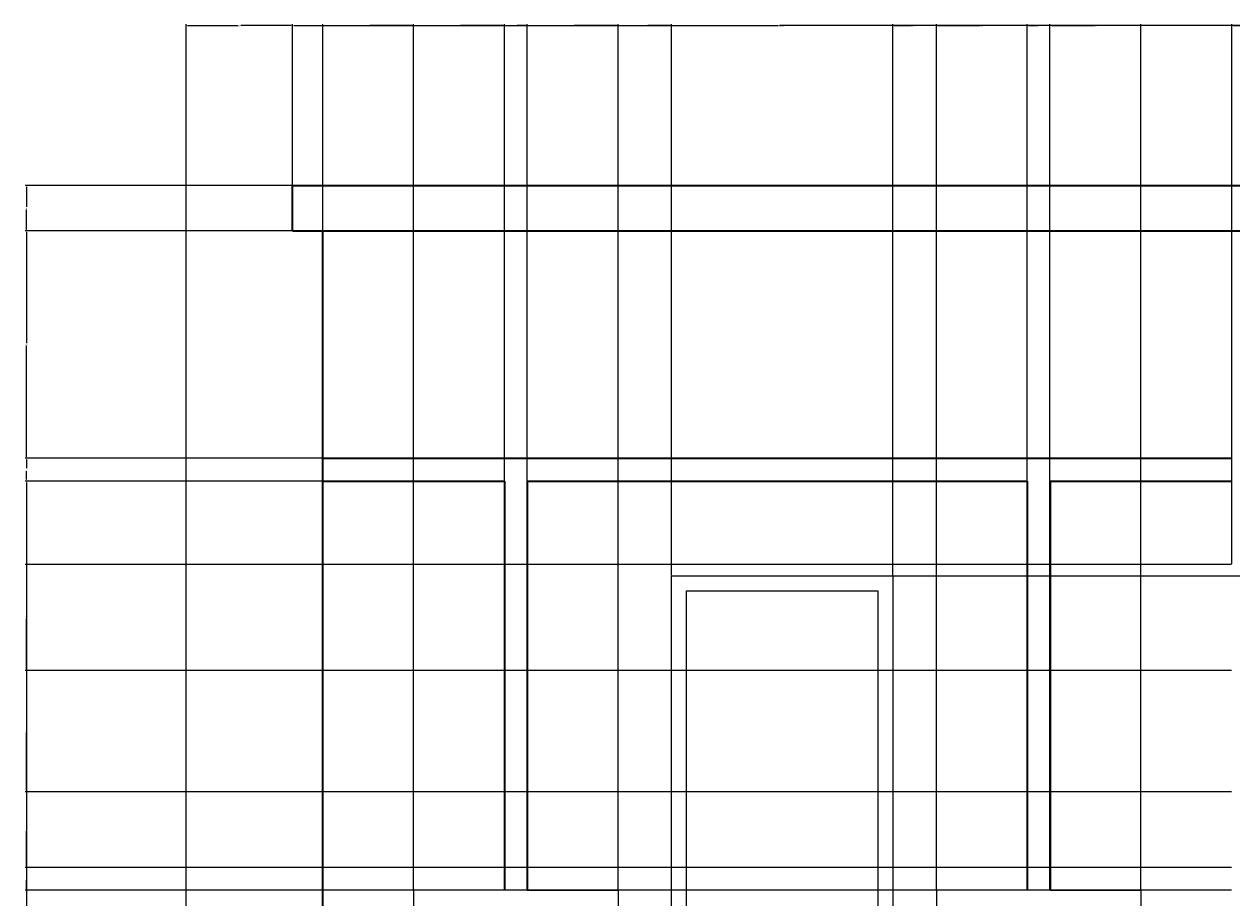
# Model space of a CAD drawing. Units: inches. Extents: x 2148 to 2587, y 1015 to 1466.
# Tile 5 of 7: x 2148 to 2307, y 1351 to 1466. Entities that reach past the tile are written whole.
import ezdxf

# ---------------------------------------------------------------- set-up
doc = ezdxf.new("R2010")
doc.units = ezdxf.units.IN
for name, color, linetype, lineweight in [('A-ANNO-DIMS', 2, 'Continuous', 18), ('A-ELEV', 7, 'Continuous', 35), ('A-GLAZ', 4, 'Continuous', 25)]:
    doc.layers.add(name, color=color, linetype=linetype, lineweight=lineweight)
doc.styles.get("Standard").update_dxf_attribs({"font": 'arial.ttf'})
doc.dimstyles.get("Standard").update_dxf_attribs({"dimtxt": 0.18, "dimasz": 0.18, "dimexe": 0.18, "dimexo": 0.0625, "dimgap": 0.09, "dimtad": 0, "dimtih": 1, "dimtoh": 1, "dimdec": 4, "dimzin": 0, "dimdsep": 46, "dimtxsty": 'Standard', "dimcen": 0.09, "dimadec": 0, "dimazin": 0, "dimtfac": 1, "dimtdec": 4, "dimtofl": 0, "dimtmove": 0, "dimatfit": 3, "dimfxl": 1, "dimtolj": 1, "dimtzin": 0, "dimarcsym": 0})

# ---------------------------------------------------------------- blocks, each defined once
blk = doc.blocks.new('*D7')
at = {"layer": 'A-ANNO-DIMS', "color": 0, "lineweight": -2, "transparency": 16777216}
for p, q in [((2169.03, 1305.54), (2169.03, 1466.02)), ((2169.21, 1465.84), (2175.82, 1465.84)), ((2182.85, 1465.84), (2176.24, 1465.84)), ((2183.03, 1444.81), (2183.03, 1466.02))]:
    blk.add_line(p, q, dxfattribs=at)
at = {"layer": 'A-ANNO-DIMS', "color": 0, "transparency": 16777216}
for points in [[(2169.21, 1465.87), (2169.21, 1465.81), (2169.03, 1465.84)], [(2182.85, 1465.87), (2182.85, 1465.81), (2183.03, 1465.84)]]:
    blk.add_solid(points, dxfattribs=at)
at = {"layer": 'Defpoints', "color": 0, "transparency": 16777216}
for p in [(2183.03, 1465.84), (2183.03, 1444.74), (2169.03, 1305.47)]:
    blk.add_point(p, dxfattribs=at)
at = {"layer": 'A-ANNO-DIMS', "color": 0, "transparency": 16777216, "insert": (2176.03, 1465.84), "char_height": 0.18, "attachment_point": 5}
blk.add_mtext('\\A1;14', dxfattribs=at)
blk = doc.blocks.new('*D8')
at = {"layer": 'A-ANNO-DIMS', "color": 0, "lineweight": -2, "transparency": 16777216}
for p, q in [((2183.03, 1444.81), (2183.03, 1466.02)), ((2183.21, 1465.84), (2246.75, 1465.84)), ((2310.85, 1465.84), (2247.31, 1465.84)), ((2311.03, 1444.81), (2311.03, 1466.02))]:
    blk.add_line(p, q, dxfattribs=at)
at = {"layer": 'A-ANNO-DIMS', "color": 0, "transparency": 16777216}
for points in [[(2183.21, 1465.87), (2183.21, 1465.81), (2183.03, 1465.84)], [(2310.85, 1465.87), (2310.85, 1465.81), (2311.03, 1465.84)]]:
    blk.add_solid(points, dxfattribs=at)
at = {"layer": 'Defpoints', "color": 0, "transparency": 16777216}
for p in [(2311.03, 1465.84), (2183.03, 1444.74), (2311.03, 1444.74)]:
    blk.add_point(p, dxfattribs=at)
at = {"layer": 'A-ANNO-DIMS', "color": 0, "transparency": 16777216, "insert": (2247.03, 1465.84), "char_height": 0.18, "attachment_point": 5}
blk.add_mtext('\\A1;128', dxfattribs=at)
blk = doc.blocks.new('*D23')
at = {"layer": 'A-ANNO-DIMS', "color": 0, "lineweight": -2, "transparency": 16777216}
for p, q in [((2186.97, 1405.74), (2147.75, 1405.74)), ((2147.93, 1405.56), (2147.93, 1286.42)), ((2147.93, 1166.92), (2147.93, 1286.06)), ((2186.97, 1166.74), (2147.75, 1166.74))]:
    blk.add_line(p, q, dxfattribs=at)
at = {"layer": 'A-ANNO-DIMS', "color": 0, "transparency": 16777216}
for points in [[(2147.9, 1405.56), (2147.96, 1405.56), (2147.93, 1405.74)], [(2147.9, 1166.92), (2147.96, 1166.92), (2147.93, 1166.74)]]:
    blk.add_solid(points, dxfattribs=at)
at = {"layer": 'Defpoints', "color": 0, "transparency": 16777216}
for p in [(2147.93, 1405.74), (2187.03, 1405.74), (2187.03, 1166.74)]:
    blk.add_point(p, dxfattribs=at)
at = {"layer": 'A-ANNO-DIMS', "color": 0, "transparency": 16777216, "insert": (2147.93, 1286.24), "char_height": 0.18, "attachment_point": 5}
blk.add_mtext('\\A1;239', dxfattribs=at)
blk = doc.blocks.new('*D24')
at = {"layer": 'A-ANNO-DIMS', "color": 0, "lineweight": -2, "transparency": 16777216}
for p, q in [((2186.97, 1408.74), (2147.75, 1408.74)), ((2147.93, 1408.56), (2147.93, 1407.42)), ((2147.93, 1405.92), (2147.93, 1407.06)), ((2186.97, 1405.74), (2147.75, 1405.74))]:
    blk.add_line(p, q, dxfattribs=at)
at = {"layer": 'A-ANNO-DIMS', "color": 0, "transparency": 16777216}
for points in [[(2147.9, 1408.56), (2147.96, 1408.56), (2147.93, 1408.74)], [(2147.9, 1405.92), (2147.96, 1405.92), (2147.93, 1405.74)]]:
    blk.add_solid(points, dxfattribs=at)
at = {"layer": 'Defpoints', "color": 0, "transparency": 16777216}
for p in [(2147.93, 1408.74), (2187.03, 1408.74), (2187.03, 1405.74)]:
    blk.add_point(p, dxfattribs=at)
at = {"layer": 'A-ANNO-DIMS', "color": 0, "transparency": 16777216, "insert": (2147.93, 1407.24), "char_height": 0.18, "attachment_point": 5}
blk.add_mtext('\\A1;3', dxfattribs=at)
blk = doc.blocks.new('*D25')
at = {"layer": 'A-ANNO-DIMS', "color": 0, "lineweight": -2, "transparency": 16777216}
for p, q in [((2182.97, 1438.74), (2147.75, 1438.74)), ((2147.93, 1438.56), (2147.93, 1423.92)), ((2147.93, 1408.92), (2147.93, 1423.56)), ((2186.97, 1408.74), (2147.75, 1408.74))]:
    blk.add_line(p, q, dxfattribs=at)
at = {"layer": 'A-ANNO-DIMS', "color": 0, "transparency": 16777216}
for points in [[(2147.9, 1438.56), (2147.96, 1438.56), (2147.93, 1438.74)], [(2147.9, 1408.92), (2147.96, 1408.92), (2147.93, 1408.74)]]:
    blk.add_solid(points, dxfattribs=at)
at = {"layer": 'Defpoints', "color": 0, "transparency": 16777216}
for p in [(2147.93, 1438.74), (2183.03, 1438.74), (2187.03, 1408.74)]:
    blk.add_point(p, dxfattribs=at)
at = {"layer": 'A-ANNO-DIMS', "color": 0, "transparency": 16777216, "insert": (2147.93, 1423.74), "char_height": 0.18, "attachment_point": 5}
blk.add_mtext('\\A1;30', dxfattribs=at)
blk = doc.blocks.new('*D26')
at = {"layer": 'A-ANNO-DIMS', "color": 0, "lineweight": -2, "transparency": 16777216}
for p, q in [((2182.97, 1444.74), (2147.75, 1444.74)), ((2147.93, 1444.56), (2147.93, 1441.92)), ((2147.93, 1438.92), (2147.93, 1441.56)), ((2182.97, 1438.74), (2147.75, 1438.74))]:
    blk.add_line(p, q, dxfattribs=at)
at = {"layer": 'A-ANNO-DIMS', "color": 0, "transparency": 16777216}
for points in [[(2147.9, 1444.56), (2147.96, 1444.56), (2147.93, 1444.74)], [(2147.9, 1438.92), (2147.96, 1438.92), (2147.93, 1438.74)]]:
    blk.add_solid(points, dxfattribs=at)
at = {"layer": 'Defpoints', "color": 0, "transparency": 16777216}
for p in [(2147.93, 1444.74), (2183.03, 1444.74), (2183.03, 1438.74)]:
    blk.add_point(p, dxfattribs=at)
at = {"layer": 'A-ANNO-DIMS', "color": 0, "transparency": 16777216, "insert": (2147.93, 1441.74), "char_height": 0.18, "attachment_point": 5}
blk.add_mtext('\\A1;6', dxfattribs=at)
blk = doc.blocks.new('*D33')
at = {"layer": 'A-ANNO-DIMS', "color": 0, "lineweight": -2, "transparency": 16777216}
for p, q in [((2307.03, 1394.81), (2307.03, 1466.02)), ((2307.21, 1465.84), (2324.89, 1465.84)), ((2343.5, 1465.84), (2325.82, 1465.84)), ((2343.68, 1366.81), (2343.68, 1466.02))]:
    blk.add_line(p, q, dxfattribs=at)
at = {"layer": 'A-ANNO-DIMS', "color": 0, "transparency": 16777216}
for points in [[(2307.21, 1465.87), (2307.21, 1465.81), (2307.03, 1465.84)], [(2343.5, 1465.87), (2343.5, 1465.81), (2343.68, 1465.84)]]:
    blk.add_solid(points, dxfattribs=at)
at = {"layer": 'Defpoints', "color": 0, "transparency": 16777216}
for p in [(2343.68, 1465.84), (2307.03, 1394.74), (2343.68, 1366.74)]:
    blk.add_point(p, dxfattribs=at)
at = {"layer": 'A-ANNO-DIMS', "color": 0, "transparency": 16777216, "insert": (2325.36, 1465.84), "char_height": 0.18, "attachment_point": 5}
blk.add_mtext('\\A1;36.645', dxfattribs=at)
blk = doc.blocks.new('*D66')
at = {"layer": 'A-ANNO-DIMS', "color": 0, "lineweight": -2, "transparency": 16777216}
for p, q in [((2306.97, 1351.74), (2147.75, 1351.74)), ((2147.93, 1351.56), (2147.93, 1349.42)), ((2147.93, 1346.92), (2147.93, 1349.06)), ((2306.97, 1346.74), (2147.75, 1346.74))]:
    blk.add_line(p, q, dxfattribs=at)
at = {"layer": 'A-ANNO-DIMS', "color": 0, "transparency": 16777216}
for points in [[(2147.9, 1351.56), (2147.96, 1351.56), (2147.93, 1351.74)], [(2147.9, 1346.92), (2147.96, 1346.92), (2147.93, 1346.74)]]:
    blk.add_solid(points, dxfattribs=at)
at = {"layer": 'Defpoints', "color": 0, "transparency": 16777216}
for p in [(2147.93, 1351.74), (2307.03, 1351.74), (2307.03, 1346.74)]:
    blk.add_point(p, dxfattribs=at)
at = {"layer": 'A-ANNO-DIMS', "color": 0, "transparency": 16777216, "insert": (2147.93, 1349.24), "char_height": 0.18, "attachment_point": 5}
blk.add_mtext('\\A1;5', dxfattribs=at)
blk = doc.blocks.new('*D67')
at = {"layer": 'A-ANNO-DIMS', "color": 0, "lineweight": -2, "transparency": 16777216}
for p, q in [((2306.97, 1354.74), (2147.75, 1354.74)), ((2147.93, 1354.56), (2147.93, 1353.42)), ((2147.93, 1351.92), (2147.93, 1353.06)), ((2306.97, 1351.74), (2147.75, 1351.74))]:
    blk.add_line(p, q, dxfattribs=at)
at = {"layer": 'A-ANNO-DIMS', "color": 0, "transparency": 16777216}
for points in [[(2147.9, 1354.56), (2147.96, 1354.56), (2147.93, 1354.74)], [(2147.9, 1351.92), (2147.96, 1351.92), (2147.93, 1351.74)]]:
    blk.add_solid(points, dxfattribs=at)
at = {"layer": 'Defpoints', "color": 0, "transparency": 16777216}
for p in [(2147.93, 1354.74), (2307.03, 1354.74), (2307.03, 1351.74)]:
    blk.add_point(p, dxfattribs=at)
at = {"layer": 'A-ANNO-DIMS', "color": 0, "transparency": 16777216, "insert": (2147.93, 1353.24), "char_height": 0.18, "attachment_point": 5}
blk.add_mtext('\\A1;3', dxfattribs=at)
blk = doc.blocks.new('*D68')
at = {"layer": 'A-ANNO-DIMS', "color": 0, "lineweight": -2, "transparency": 16777216}
for p, q in [((2306.97, 1364.74), (2147.75, 1364.74)), ((2147.93, 1364.56), (2147.93, 1359.92)), ((2147.93, 1354.92), (2147.93, 1359.56)), ((2306.97, 1354.74), (2147.75, 1354.74))]:
    blk.add_line(p, q, dxfattribs=at)
at = {"layer": 'A-ANNO-DIMS', "color": 0, "transparency": 16777216}
for points in [[(2147.9, 1364.56), (2147.96, 1364.56), (2147.93, 1364.74)], [(2147.9, 1354.92), (2147.96, 1354.92), (2147.93, 1354.74)]]:
    blk.add_solid(points, dxfattribs=at)
at = {"layer": 'Defpoints', "color": 0, "transparency": 16777216}
for p in [(2147.93, 1364.74), (2307.03, 1364.74), (2307.03, 1354.74)]:
    blk.add_point(p, dxfattribs=at)
at = {"layer": 'A-ANNO-DIMS', "color": 0, "transparency": 16777216, "insert": (2147.93, 1359.74), "char_height": 0.18, "attachment_point": 5}
blk.add_mtext('\\A1;10', dxfattribs=at)
blk = doc.blocks.new('*D69')
at = {"layer": 'A-ANNO-DIMS', "color": 0, "lineweight": -2, "transparency": 16777216}
for p, q in [((2306.97, 1380.74), (2147.75, 1380.74)), ((2147.93, 1380.56), (2147.93, 1372.92)), ((2147.93, 1364.92), (2147.93, 1372.56)), ((2306.97, 1364.74), (2147.75, 1364.74))]:
    blk.add_line(p, q, dxfattribs=at)
at = {"layer": 'A-ANNO-DIMS', "color": 0, "transparency": 16777216}
for points in [[(2147.9, 1380.56), (2147.96, 1380.56), (2147.93, 1380.74)], [(2147.9, 1364.92), (2147.96, 1364.92), (2147.93, 1364.74)]]:
    blk.add_solid(points, dxfattribs=at)
at = {"layer": 'Defpoints', "color": 0, "transparency": 16777216}
for p in [(2147.93, 1380.74), (2307.03, 1380.74), (2307.03, 1364.74)]:
    blk.add_point(p, dxfattribs=at)
at = {"layer": 'A-ANNO-DIMS', "color": 0, "transparency": 16777216, "insert": (2147.93, 1372.74), "char_height": 0.18, "attachment_point": 5}
blk.add_mtext('\\A1;16', dxfattribs=at)
blk = doc.blocks.new('*D70')
at = {"layer": 'A-ANNO-DIMS', "color": 0, "lineweight": -2, "transparency": 16777216}
for p, q in [((2306.97, 1394.74), (2147.75, 1394.74)), ((2147.93, 1394.56), (2147.93, 1387.92)), ((2147.93, 1380.92), (2147.93, 1387.56)), ((2306.97, 1380.74), (2147.75, 1380.74))]:
    blk.add_line(p, q, dxfattribs=at)
at = {"layer": 'A-ANNO-DIMS', "color": 0, "transparency": 16777216}
for points in [[(2147.9, 1394.56), (2147.96, 1394.56), (2147.93, 1394.74)], [(2147.9, 1380.92), (2147.96, 1380.92), (2147.93, 1380.74)]]:
    blk.add_solid(points, dxfattribs=at)
at = {"layer": 'Defpoints', "color": 0, "transparency": 16777216}
for p in [(2147.93, 1394.74), (2307.03, 1394.74), (2307.03, 1380.74)]:
    blk.add_point(p, dxfattribs=at)
at = {"layer": 'A-ANNO-DIMS', "color": 0, "transparency": 16777216, "insert": (2147.93, 1387.74), "char_height": 0.18, "attachment_point": 5}
blk.add_mtext('\\A1;14', dxfattribs=at)
blk = doc.blocks.new('*D73')
at = {"layer": 'A-ANNO-DIMS', "color": 0, "lineweight": -2, "transparency": 16777216}
for p, q in [((2187.03, 1166.81), (2187.03, 1466.02)), ((2187.21, 1465.84), (2192.82, 1465.84)), ((2198.85, 1465.84), (2193.24, 1465.84)), ((2199.03, 1351.81), (2199.03, 1466.02))]:
    blk.add_line(p, q, dxfattribs=at)
at = {"layer": 'A-ANNO-DIMS', "color": 0, "transparency": 16777216}
for points in [[(2187.21, 1465.87), (2187.21, 1465.81), (2187.03, 1465.84)], [(2198.85, 1465.87), (2198.85, 1465.81), (2199.03, 1465.84)]]:
    blk.add_solid(points, dxfattribs=at)
at = {"layer": 'Defpoints', "color": 0, "transparency": 16777216}
for p in [(2199.03, 1465.84), (2199.03, 1351.74), (2187.03, 1166.74)]:
    blk.add_point(p, dxfattribs=at)
at = {"layer": 'A-ANNO-DIMS', "color": 0, "transparency": 16777216, "insert": (2193.03, 1465.84), "char_height": 0.18, "attachment_point": 5}
blk.add_mtext('\\A1;12', dxfattribs=at)
blk = doc.blocks.new('*D74')
at = {"layer": 'A-ANNO-DIMS', "color": 0, "lineweight": -2, "transparency": 16777216}
for p, q in [((2199.03, 1351.81), (2199.03, 1466.02)), ((2199.21, 1465.84), (2204.82, 1465.84)), ((2210.85, 1465.84), (2205.24, 1465.84)), ((2211.03, 1351.81), (2211.03, 1466.02))]:
    blk.add_line(p, q, dxfattribs=at)
at = {"layer": 'A-ANNO-DIMS', "color": 0, "transparency": 16777216}
for points in [[(2199.21, 1465.87), (2199.21, 1465.81), (2199.03, 1465.84)], [(2210.85, 1465.87), (2210.85, 1465.81), (2211.03, 1465.84)]]:
    blk.add_solid(points, dxfattribs=at)
at = {"layer": 'Defpoints', "color": 0, "transparency": 16777216}
for p in [(2211.03, 1465.84), (2199.03, 1351.74), (2211.03, 1351.74)]:
    blk.add_point(p, dxfattribs=at)
at = {"layer": 'A-ANNO-DIMS', "color": 0, "transparency": 16777216, "insert": (2205.03, 1465.84), "char_height": 0.18, "attachment_point": 5}
blk.add_mtext('\\A1;12', dxfattribs=at)
blk = doc.blocks.new('*D75')
at = {"layer": 'A-ANNO-DIMS', "color": 0, "lineweight": -2, "transparency": 16777216}
for p, q in [((2211.03, 1351.81), (2211.03, 1466.02)), ((2211.21, 1465.84), (2212.39, 1465.84)), ((2213.85, 1465.84), (2212.68, 1465.84)), ((2214.03, 1351.81), (2214.03, 1466.02))]:
    blk.add_line(p, q, dxfattribs=at)
at = {"layer": 'A-ANNO-DIMS', "color": 0, "transparency": 16777216}
for points in [[(2211.21, 1465.87), (2211.21, 1465.81), (2211.03, 1465.84)], [(2213.85, 1465.87), (2213.85, 1465.81), (2214.03, 1465.84)]]:
    blk.add_solid(points, dxfattribs=at)
at = {"layer": 'Defpoints', "color": 0, "transparency": 16777216}
for p in [(2214.03, 1465.84), (2211.03, 1351.74), (2214.03, 1351.74)]:
    blk.add_point(p, dxfattribs=at)
at = {"layer": 'A-ANNO-DIMS', "color": 0, "transparency": 16777216, "insert": (2212.53, 1465.84), "char_height": 0.18, "attachment_point": 5}
blk.add_mtext('\\A1;3', dxfattribs=at)
blk = doc.blocks.new('*D76')
at = {"layer": 'A-ANNO-DIMS', "color": 0, "lineweight": -2, "transparency": 16777216}
for p, q in [((2214.03, 1351.81), (2214.03, 1466.02)), ((2214.21, 1465.84), (2219.82, 1465.84)), ((2225.85, 1465.84), (2220.24, 1465.84)), ((2226.03, 1351.81), (2226.03, 1466.02))]:
    blk.add_line(p, q, dxfattribs=at)
at = {"layer": 'A-ANNO-DIMS', "color": 0, "transparency": 16777216}
for points in [[(2214.21, 1465.87), (2214.21, 1465.81), (2214.03, 1465.84)], [(2225.85, 1465.87), (2225.85, 1465.81), (2226.03, 1465.84)]]:
    blk.add_solid(points, dxfattribs=at)
at = {"layer": 'Defpoints', "color": 0, "transparency": 16777216}
for p in [(2226.03, 1465.84), (2214.03, 1351.74), (2226.03, 1351.74)]:
    blk.add_point(p, dxfattribs=at)
at = {"layer": 'A-ANNO-DIMS', "color": 0, "transparency": 16777216, "insert": (2220.03, 1465.84), "char_height": 0.18, "attachment_point": 5}
blk.add_mtext('\\A1;12', dxfattribs=at)
blk = doc.blocks.new('*D77')
at = {"layer": 'A-ANNO-DIMS', "color": 0, "lineweight": -2, "transparency": 16777216}
for p, q in [((2226.03, 1351.81), (2226.03, 1466.02)), ((2226.21, 1465.84), (2229.15, 1465.84)), ((2232.88, 1465.84), (2229.94, 1465.84)), ((2233.06, 1393.3), (2233.06, 1466.02))]:
    blk.add_line(p, q, dxfattribs=at)
at = {"layer": 'A-ANNO-DIMS', "color": 0, "transparency": 16777216}
for points in [[(2226.21, 1465.87), (2226.21, 1465.81), (2226.03, 1465.84)], [(2232.88, 1465.87), (2232.88, 1465.81), (2233.06, 1465.84)]]:
    blk.add_solid(points, dxfattribs=at)
at = {"layer": 'Defpoints', "color": 0, "transparency": 16777216}
for p in [(2233.06, 1465.84), (2233.06, 1393.24), (2226.03, 1351.74)]:
    blk.add_point(p, dxfattribs=at)
at = {"layer": 'A-ANNO-DIMS', "color": 0, "transparency": 16777216, "insert": (2229.55, 1465.84), "char_height": 0.18, "attachment_point": 5}
blk.add_mtext('\\A1;7.026', dxfattribs=at)
blk = doc.blocks.new('*D78')
at = {"layer": 'A-ANNO-DIMS', "color": 0, "lineweight": -2, "transparency": 16777216}
for p, q in [((2233.06, 1393.3), (2233.06, 1466.02)), ((2233.24, 1465.84), (2247.21, 1465.84)), ((2262.11, 1465.84), (2248.14, 1465.84)), ((2262.29, 1393.3), (2262.29, 1466.02))]:
    blk.add_line(p, q, dxfattribs=at)
at = {"layer": 'A-ANNO-DIMS', "color": 0, "transparency": 16777216}
for points in [[(2233.24, 1465.87), (2233.24, 1465.81), (2233.06, 1465.84)], [(2262.11, 1465.87), (2262.11, 1465.81), (2262.29, 1465.84)]]:
    blk.add_solid(points, dxfattribs=at)
at = {"layer": 'Defpoints', "color": 0, "transparency": 16777216}
for p in [(2262.29, 1465.84), (2233.06, 1393.24), (2262.29, 1393.24)]:
    blk.add_point(p, dxfattribs=at)
at = {"layer": 'A-ANNO-DIMS', "color": 0, "transparency": 16777216, "insert": (2247.67, 1465.84), "char_height": 0.18, "attachment_point": 5}
blk.add_mtext('\\A1;29.227', dxfattribs=at)
blk = doc.blocks.new('*D79')
at = {"layer": 'A-ANNO-DIMS', "color": 0, "lineweight": -2, "transparency": 16777216}
for p, q in [((2262.29, 1393.3), (2262.29, 1466.02)), ((2262.47, 1465.84), (2264.77, 1465.84)), ((2267.85, 1465.84), (2265.55, 1465.84)), ((2268.03, 1351.81), (2268.03, 1466.02))]:
    blk.add_line(p, q, dxfattribs=at)
at = {"layer": 'A-ANNO-DIMS', "color": 0, "transparency": 16777216}
for points in [[(2262.47, 1465.87), (2262.47, 1465.81), (2262.29, 1465.84)], [(2267.85, 1465.87), (2267.85, 1465.81), (2268.03, 1465.84)]]:
    blk.add_solid(points, dxfattribs=at)
at = {"layer": 'Defpoints', "color": 0, "transparency": 16777216}
for p in [(2268.03, 1465.84), (2262.29, 1393.24), (2268.03, 1351.74)]:
    blk.add_point(p, dxfattribs=at)
at = {"layer": 'A-ANNO-DIMS', "color": 0, "transparency": 16777216, "insert": (2265.16, 1465.84), "char_height": 0.18, "attachment_point": 5}
blk.add_mtext('\\A1;5.747', dxfattribs=at)
blk = doc.blocks.new('*D80')
at = {"layer": 'A-ANNO-DIMS', "color": 0, "lineweight": -2, "transparency": 16777216}
for p, q in [((2268.03, 1351.81), (2268.03, 1466.02)), ((2268.21, 1465.84), (2273.82, 1465.84)), ((2279.85, 1465.84), (2274.24, 1465.84)), ((2280.03, 1351.81), (2280.03, 1466.02))]:
    blk.add_line(p, q, dxfattribs=at)
at = {"layer": 'A-ANNO-DIMS', "color": 0, "transparency": 16777216}
for points in [[(2268.21, 1465.87), (2268.21, 1465.81), (2268.03, 1465.84)], [(2279.85, 1465.87), (2279.85, 1465.81), (2280.03, 1465.84)]]:
    blk.add_solid(points, dxfattribs=at)
at = {"layer": 'Defpoints', "color": 0, "transparency": 16777216}
for p in [(2280.03, 1465.84), (2268.03, 1351.74), (2280.03, 1351.74)]:
    blk.add_point(p, dxfattribs=at)
at = {"layer": 'A-ANNO-DIMS', "color": 0, "transparency": 16777216, "insert": (2274.03, 1465.84), "char_height": 0.18, "attachment_point": 5}
blk.add_mtext('\\A1;12', dxfattribs=at)
blk = doc.blocks.new('*D81')
at = {"layer": 'A-ANNO-DIMS', "color": 0, "lineweight": -2, "transparency": 16777216}
for p, q in [((2280.03, 1351.81), (2280.03, 1466.02)), ((2280.21, 1465.84), (2281.39, 1465.84)), ((2282.85, 1465.84), (2281.68, 1465.84)), ((2283.03, 1351.81), (2283.03, 1466.02))]:
    blk.add_line(p, q, dxfattribs=at)
at = {"layer": 'A-ANNO-DIMS', "color": 0, "transparency": 16777216}
for points in [[(2280.21, 1465.87), (2280.21, 1465.81), (2280.03, 1465.84)], [(2282.85, 1465.87), (2282.85, 1465.81), (2283.03, 1465.84)]]:
    blk.add_solid(points, dxfattribs=at)
at = {"layer": 'Defpoints', "color": 0, "transparency": 16777216}
for p in [(2283.03, 1465.84), (2280.03, 1351.74), (2283.03, 1351.74)]:
    blk.add_point(p, dxfattribs=at)
at = {"layer": 'A-ANNO-DIMS', "color": 0, "transparency": 16777216, "insert": (2281.53, 1465.84), "char_height": 0.18, "attachment_point": 5}
blk.add_mtext('\\A1;3', dxfattribs=at)
blk = doc.blocks.new('*D82')
at = {"layer": 'A-ANNO-DIMS', "color": 0, "lineweight": -2, "transparency": 16777216}
for p, q in [((2283.03, 1351.81), (2283.03, 1466.02)), ((2283.21, 1465.84), (2288.82, 1465.84)), ((2294.85, 1465.84), (2289.24, 1465.84)), ((2295.03, 1351.81), (2295.03, 1466.02))]:
    blk.add_line(p, q, dxfattribs=at)
at = {"layer": 'A-ANNO-DIMS', "color": 0, "transparency": 16777216}
for points in [[(2283.21, 1465.87), (2283.21, 1465.81), (2283.03, 1465.84)], [(2294.85, 1465.87), (2294.85, 1465.81), (2295.03, 1465.84)]]:
    blk.add_solid(points, dxfattribs=at)
at = {"layer": 'Defpoints', "color": 0, "transparency": 16777216}
for p in [(2295.03, 1465.84), (2283.03, 1351.74), (2295.03, 1351.74)]:
    blk.add_point(p, dxfattribs=at)
at = {"layer": 'A-ANNO-DIMS', "color": 0, "transparency": 16777216, "insert": (2289.03, 1465.84), "char_height": 0.18, "attachment_point": 5}
blk.add_mtext('\\A1;12', dxfattribs=at)
blk = doc.blocks.new('*D91')
at = {"layer": 'A-ANNO-DIMS', "color": 0, "lineweight": -2, "transparency": 16777216}
for p, q in [((2198.97, 1351.74), (2147.75, 1351.74)), ((2147.93, 1351.56), (2147.93, 1269.82)), ((2147.93, 1187.71), (2147.93, 1269.45)), ((2201.43, 1187.53), (2147.75, 1187.53))]:
    blk.add_line(p, q, dxfattribs=at)
at = {"layer": 'A-ANNO-DIMS', "color": 0, "transparency": 16777216}
for points in [[(2147.9, 1351.56), (2147.96, 1351.56), (2147.93, 1351.74)], [(2147.9, 1187.71), (2147.96, 1187.71), (2147.93, 1187.53)]]:
    blk.add_solid(points, dxfattribs=at)
at = {"layer": 'Defpoints', "color": 0, "transparency": 16777216}
for p in [(2147.93, 1351.74), (2199.03, 1351.74), (2201.49, 1187.53)]:
    blk.add_point(p, dxfattribs=at)
at = {"layer": 'A-ANNO-DIMS', "color": 0, "transparency": 16777216, "insert": (2147.93, 1269.64), "char_height": 0.18, "attachment_point": 5}
blk.add_mtext('\\A1;164.2', dxfattribs=at)
blk = doc.blocks.new('*D97')
at = {"layer": 'A-ANNO-DIMS', "color": 0, "lineweight": -2, "transparency": 16777216}
for p, q in [((2262.35, 1393.24), (2586.31, 1393.24)), ((2586.13, 1393.06), (2586.13, 1369.55)), ((2586.13, 1345.67), (2586.13, 1369.18)), ((2260.35, 1345.49), (2586.31, 1345.49))]:
    blk.add_line(p, q, dxfattribs=at)
at = {"layer": 'A-ANNO-DIMS', "color": 0, "transparency": 16777216}
for points in [[(2586.1, 1393.06), (2586.16, 1393.06), (2586.13, 1393.24)], [(2586.1, 1345.67), (2586.16, 1345.67), (2586.13, 1345.49)]]:
    blk.add_solid(points, dxfattribs=at)
at = {"layer": 'Defpoints', "color": 0, "transparency": 16777216}
for p in [(2262.29, 1393.24), (2586.13, 1393.24), (2260.29, 1345.49)]:
    blk.add_point(p, dxfattribs=at)
at = {"layer": 'A-ANNO-DIMS', "color": 0, "transparency": 16777216, "insert": (2586.13, 1369.36), "char_height": 0.18, "attachment_point": 5}
blk.add_mtext('\\A1;47.75', dxfattribs=at)

msp = doc.modelspace()

# ---------------------------------------------------------------- linework, layer by layer
at = {"layer": 'A-ELEV'}
for p, q in [((2183.0343, 1438.7427), (2183.0343, 1444.7427)), ((2183.0343, 1444.7427), (2311.0343, 1444.7427)), ((2183.0343, 1438.7427), (2311.0343, 1438.7427)), ((2187.0343, 1048.7427), (2187.0343, 1438.7427)), ((2187.0343, 1408.7427), (2307.0343, 1408.7427)), ((2187.0343, 1405.7427), (2211.0343, 1405.7427)), ((2211.0343, 1405.7427), (2211.0343, 1351.7427)), ((2214.0343, 1405.7427), (2214.0343, 1351.7427)), ((2214.0343, 1405.7427), (2280.0343, 1405.7427)), ((2280.0343, 1405.7427), (2280.0343, 1351.7427)), ((2283.0343, 1405.7427), (2283.0343, 1351.7427)), ((2283.0343, 1405.7427), (2307.0343, 1405.7427))]:
    msp.add_line(p, q, dxfattribs=at)
at = {"layer": 'A-GLAZ'}
for p, q in [((2211.0343, 1351.7427), (2199.0343, 1351.7427)), ((2199.0343, 1351.7427), (2199.0343, 1174.7427)), ((2226.0343, 1351.7427), (2199.0343, 1351.7427)), ((2214.0343, 1351.7427), (2226.0343, 1351.7427)), ((2226.0343, 1351.7427), (2226.0343, 1174.7427)), ((2295.0343, 1351.7427), (2268.0343, 1351.7427)), ((2280.0343, 1351.7427), (2268.0343, 1351.7427)), ((2268.0343, 1351.7427), (2268.0343, 1174.7427)), ((2283.0343, 1351.7427), (2295.0343, 1351.7427)), ((2295.0343, 1351.7427), (2295.0343, 1174.7427))]:
    msp.add_line(p, q, dxfattribs=at)
for points in [[(2262.287, 1197.738), (2233.0602, 1197.738), (2233.0602, 1393.2389), (2262.287, 1393.2389)], [(2260.287, 1199.738), (2235.0602, 1199.738), (2235.0602, 1391.2389), (2260.287, 1391.2389)]]:
    msp.add_lwpolyline(points, close=True, dxfattribs=at)

# ---------------------------------------------------------------- dimensions: what is measured, and where the dimension line sits
at = {"layer": 'A-ANNO-DIMS'}
for base, p1, p2, override, picture, middle in [((2183.0343, 1465.8427), (2169.0343, 1305.4734), (2183.0343, 1444.7427), {"dimdec": 0, "dimlfac": 1, "dimrnd": 0, "dimzin": 0, "dimdsep": 46, "dimlunit": 2}, '*D7', (2176.0343, 1465.8427)), ((2311.0343, 1465.8427), (2183.0343, 1444.7427), (2311.0343, 1444.7427), {"dimdec": 0, "dimlfac": 1, "dimrnd": 0, "dimzin": 0, "dimdsep": 46, "dimlunit": 2}, '*D8', (2247.0343, 1465.8427)), ((2199.0343, 1465.8427), (2187.0343, 1166.7427), (2199.0343, 1351.7427), {"dimdec": 0, "dimlfac": 1, "dimrnd": 0, "dimzin": 0, "dimdsep": 46, "dimlunit": 2}, '*D73', (2193.0343, 1465.8427)), ((2211.0343, 1465.8427), (2199.0343, 1351.7427), (2211.0343, 1351.7427), {"dimdec": 0, "dimlfac": 1, "dimrnd": 0, "dimzin": 0, "dimdsep": 46, "dimlunit": 2}, '*D74', (2205.0343, 1465.8427)), ((2214.0343, 1465.8427), (2211.0343, 1351.7427), (2214.0343, 1351.7427), {"dimdec": 0, "dimlfac": 1, "dimrnd": 0, "dimzin": 0, "dimdsep": 46, "dimlunit": 2}, '*D75', (2212.5343, 1465.8427)), ((2226.0343, 1465.8427), (2214.0343, 1351.7427), (2226.0343, 1351.7427), {"dimdec": 0, "dimlfac": 1, "dimrnd": 0, "dimzin": 0, "dimdsep": 46, "dimlunit": 2}, '*D76', (2220.0343, 1465.8427)), ((2233.0602, 1465.8427), (2226.0343, 1351.7427), (2233.0602, 1393.2389), {"dimdec": 3, "dimlfac": 1, "dimrnd": 0, "dimzin": 0, "dimdsep": 46, "dimlunit": 2}, '*D77', (2229.5472, 1465.8427)), ((2262.287, 1465.8427), (2233.0602, 1393.2389), (2262.287, 1393.2389), {"dimdec": 3, "dimlfac": 1, "dimrnd": 0, "dimzin": 0, "dimdsep": 46, "dimlunit": 2}, '*D78', (2247.6736, 1465.8427)), ((2268.0343, 1465.8427), (2262.287, 1393.2389), (2268.0343, 1351.7427), {"dimdec": 3, "dimlfac": 1, "dimrnd": 0, "dimzin": 0, "dimdsep": 46, "dimlunit": 2}, '*D79', (2265.1606, 1465.8427)), ((2280.0343, 1465.8427), (2268.0343, 1351.7427), (2280.0343, 1351.7427), {"dimdec": 0, "dimlfac": 1, "dimrnd": 0, "dimzin": 0, "dimdsep": 46, "dimlunit": 2}, '*D80', (2274.0343, 1465.8427)), ((2283.0343, 1465.8427), (2280.0343, 1351.7427), (2283.0343, 1351.7427), {"dimdec": 0, "dimlfac": 1, "dimrnd": 0, "dimzin": 0, "dimdsep": 46, "dimlunit": 2}, '*D81', (2281.5343, 1465.8427)), ((2295.0343, 1465.8427), (2283.0343, 1351.7427), (2295.0343, 1351.7427), {"dimdec": 0, "dimlfac": 1, "dimrnd": 0, "dimzin": 0, "dimdsep": 46, "dimlunit": 2}, '*D82', (2289.0343, 1465.8427)), ((2343.6794, 1465.8427), (2307.0343, 1394.7427), (2343.6794, 1366.7427), {"dimdec": 3, "dimlfac": 1, "dimrnd": 0, "dimzin": 0, "dimdsep": 46, "dimlunit": 2}, '*D33', (2325.3568, 1465.8427))]:
    dim = msp.add_linear_dim(base=base, p1=p1, p2=p2, dimstyle='Standard', override=override, dxfattribs=at)
    dim.commit()
    dim.dimension.update_dxf_attribs({"geometry": picture, "text_midpoint": middle})
for base, p1, p2, override, picture, middle in [((2147.9343, 1444.7427), (2183.0343, 1438.7427), (2183.0343, 1444.7427), {"dimdec": 0, "dimlfac": 1, "dimrnd": 0, "dimzin": 0, "dimdsep": 46, "dimlunit": 2}, '*D26', (2147.9343, 1441.7427)), ((2147.9343, 1438.7427), (2187.0343, 1408.7427), (2183.0343, 1438.7427), {"dimdec": 0, "dimlfac": 1, "dimrnd": 0, "dimzin": 0, "dimdsep": 46, "dimlunit": 2}, '*D25', (2147.9343, 1423.7427)), ((2147.9343, 1408.7427), (2187.0343, 1405.7427), (2187.0343, 1408.7427), {"dimdec": 0, "dimlfac": 1, "dimrnd": 0, "dimzin": 0, "dimdsep": 46, "dimlunit": 2}, '*D24', (2147.9343, 1407.2427)), ((2147.9343, 1405.7427), (2187.0343, 1166.7427), (2187.0343, 1405.7427), {"dimdec": 0, "dimlfac": 1, "dimrnd": 0, "dimzin": 0, "dimdsep": 46, "dimlunit": 2}, '*D23', (2147.9343, 1286.2427)), ((2147.9343, 1394.7427), (2307.0343, 1380.7427), (2307.0343, 1394.7427), {"dimdec": 0, "dimlfac": 1, "dimrnd": 0, "dimzin": 0, "dimdsep": 46, "dimlunit": 2}, '*D70', (2147.9343, 1387.7427)), ((2586.1343, 1393.2389), (2260.287, 1345.4885), (2262.287, 1393.2389), {"dimdec": 2, "dimlfac": 1, "dimrnd": 0, "dimzin": 0, "dimdsep": 46, "dimlunit": 2}, '*D97', (2586.1343, 1369.3637)), ((2147.9343, 1380.7427), (2307.0343, 1364.7427), (2307.0343, 1380.7427), {"dimdec": 0, "dimlfac": 1, "dimrnd": 0, "dimzin": 0, "dimdsep": 46, "dimlunit": 2}, '*D69', (2147.9343, 1372.7427)), ((2147.9343, 1364.7427), (2307.0343, 1354.7427), (2307.0343, 1364.7427), {"dimdec": 0, "dimlfac": 1, "dimrnd": 0, "dimzin": 0, "dimdsep": 46, "dimlunit": 2}, '*D68', (2147.9343, 1359.7427)), ((2147.9343, 1354.7427), (2307.0343, 1351.7427), (2307.0343, 1354.7427), {"dimdec": 0, "dimlfac": 1, "dimrnd": 0, "dimzin": 0, "dimdsep": 46, "dimlunit": 2}, '*D67', (2147.9343, 1353.2427)), ((2147.9343, 1351.7427), (2201.4949, 1187.5293), (2199.0343, 1351.7427), {"dimdec": 1, "dimlfac": 1, "dimrnd": 0, "dimzin": 0, "dimdsep": 46, "dimlunit": 2}, '*D91', (2147.9343, 1269.636)), ((2147.9343, 1351.7427), (2307.0343, 1346.7427), (2307.0343, 1351.7427), {"dimdec": 0, "dimlfac": 1, "dimrnd": 0, "dimzin": 0, "dimdsep": 46, "dimlunit": 2}, '*D66', (2147.9343, 1349.2427))]:
    dim = msp.add_linear_dim(base=base, p1=p1, p2=p2, angle=90, dimstyle='Standard', override=override, dxfattribs=at)
    dim.commit()
    dim.dimension.update_dxf_attribs({"geometry": picture, "text_midpoint": middle})

doc.saveas('drawing.dxf')
